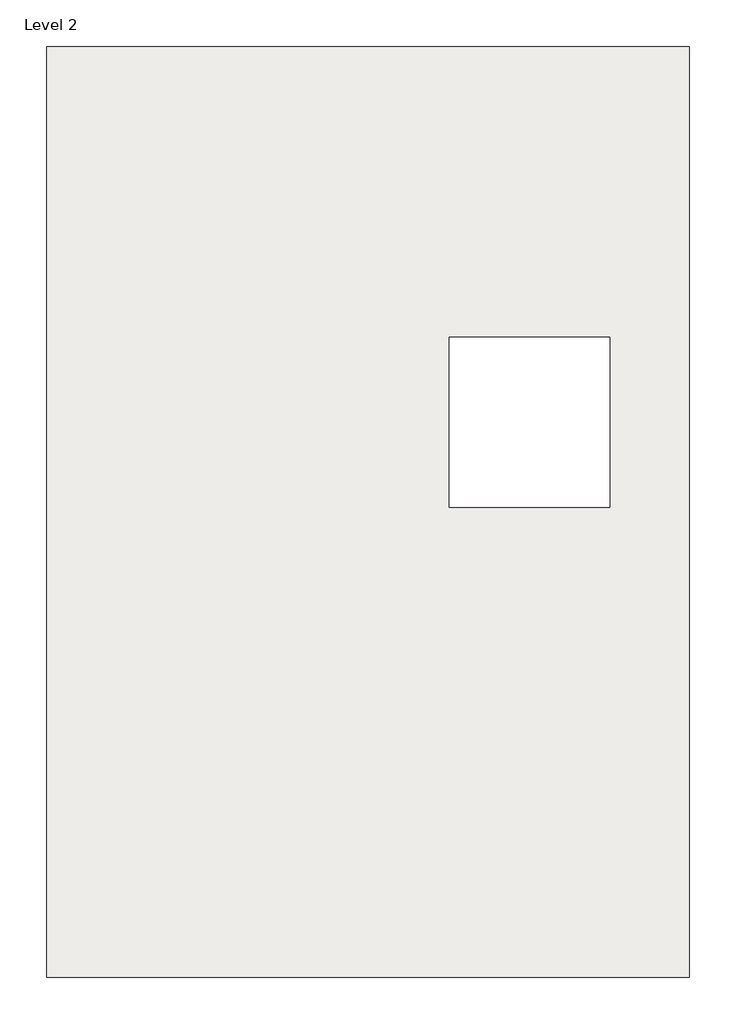
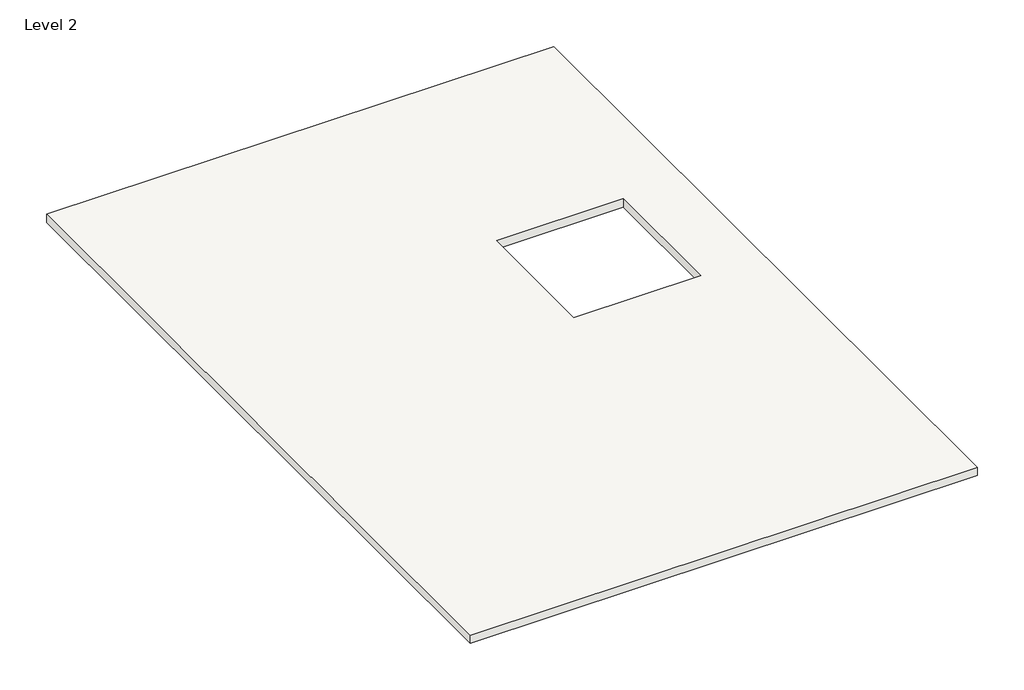
# One storey: 1 roof.
"""IFC4 building model written with IfcOpenShell, lengths in millimetres."""

from ifc_helpers import new_model, si_unit, frame, origin, place, context, project, spatial, polyline, outline, extrude, element, save

model = new_model("IFC4")

# Units and contexts
model_context = context("Model", 3, world=origin())
ifc_project = project(units=[si_unit("LENGTHUNIT", "METRE", prefix="MILLI")], contexts=[model_context])

# Site, building, storey
site = spatial("IfcSite", under=ifc_project)
building = spatial("IfcBuilding", under=site)
storey = spatial("IfcBuildingStorey", under=building, Name="Level 2", Elevation=3048.0)

# Roof
placement = place(None, origin())
element("IfcRoof", 1, ObjectType="Generic - 12\"", at=placement, inside=storey, context=model_context, shape_type="SweptSolid", body=[
    extrude(outline(polyline([(3164.3584916, 6938.9935985), (3164.3584916, -5862.6064015), (-5674.8415084, -5862.6064015), (-5674.8415084, 6938.9935985), (3164.3584916, 6938.9935985)]), holes=[polyline([(2072.9441983, 2938.4935985), (-137.6415084, 2938.4935985), (-137.6415084, 601.6935985), (2072.9441983, 601.6935985), (2072.9441983, 2938.4935985)])]), frame((0.0, 0.0, 3048.0), z_axis=(0.0, 0.0, 1.0), x_axis=(1.0, 0.0, 0.0)), (0.0, 0.0, 1.0), 152.4),
])

save(model, "model.ifc")

# Revit data of these elements
# Type "Generic - 12\""
#   Assembly Code = "B1020"
#   Layers, outside or top first: 0' - 6" no material (function 1)
# Element 1 (IfcRoof, "Generic - 12\"")
#   built-in parameter 1001705 = 10.5 (stored number, unit not read)
#   built-in parameter 1001710 = 33615
#   Phase Created = New Construction
#   Materials on its faces: "Default Roof"
# Materials
#   "Default Roof": colour RGB 88 101 114, transparency 0, Cost = 0
